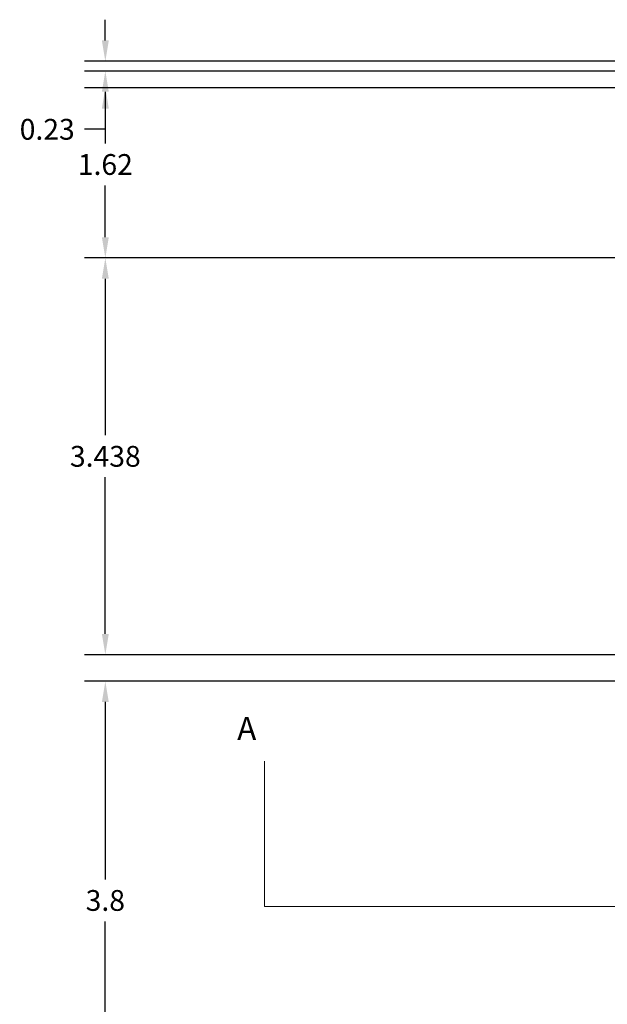
# Model space of a CAD drawing. Units: metres. Extents: x 2031 to 2061.8, y 1886.4 to 1909.8.
# Tile 4 of 10: x 2031 to 2036.1, y 1896.6 to 1905.1. Entities that reach past the tile are written whole.
import ezdxf

# ---------------------------------------------------------------- set-up
doc = ezdxf.new("R2010")
doc.units = ezdxf.units.M
doc.layers.add('A-ANNO-DIMS', color=2, linetype='Continuous', lineweight=18)
doc.layers.add('A-ANNO-SYMB', color=7, linetype='Continuous', lineweight=18)
doc.styles.get("Standard").update_dxf_attribs({"font": 'arial.ttf'})
doc.dimstyles.get("Standard").update_dxf_attribs({"dimtxt": 0.18, "dimasz": 0.18, "dimexe": 0.18, "dimexo": 0.0625, "dimgap": 0.09, "dimtad": 0, "dimtih": 1, "dimtoh": 1, "dimdec": 4, "dimzin": 0, "dimdsep": 46, "dimtxsty": 'Standard', "dimcen": 0.09, "dimadec": 0, "dimazin": 0, "dimtfac": 1, "dimtdec": 4, "dimtofl": 0, "dimtmove": 0, "dimatfit": 3, "dimfxl": 1, "dimtolj": 1, "dimtzin": 0, "dimarcsym": 0})

# ---------------------------------------------------------------- blocks, each defined once
blk = doc.blocks.new('*D51')
at = {"layer": 'A-ANNO-DIMS', "color": 0, "lineweight": -2, "transparency": 16777216}
for p, q in [((2036.9007, 1899.3712), (2031.5648, 1899.3712)), ((2031.7448, 1899.1912), (2031.7448, 1897.6532)), ((2031.7448, 1895.7512), (2031.7448, 1897.2892)), ((2036.9007, 1895.5712), (2031.5648, 1895.5712))]:
    blk.add_line(p, q, dxfattribs=at)
at = {"layer": 'A-ANNO-DIMS', "color": 0, "transparency": 16777216}
for points in [[(2031.7148, 1899.1912), (2031.7748, 1899.1912), (2031.7448, 1899.3712)], [(2031.7148, 1895.7512), (2031.7748, 1895.7512), (2031.7448, 1895.5712)]]:
    blk.add_solid(points, dxfattribs=at)
at = {"layer": 'Defpoints', "color": 0, "transparency": 16777216}
for p in [(2031.7448, 1899.3712), (2036.9632, 1899.3712), (2036.9632, 1895.5712)]:
    blk.add_point(p, dxfattribs=at)
at = {"layer": 'A-ANNO-DIMS', "color": 0, "transparency": 16777216, "insert": (2031.7448, 1897.4712), "char_height": 0.18, "attachment_point": 5}
blk.add_mtext('\\A1;3.8', dxfattribs=at)
blk = doc.blocks.new('*D52')
at = {"layer": 'A-ANNO-DIMS', "color": 0, "lineweight": -2, "transparency": 16777216}
for p, q in [((2036.1714, 1903.039), (2031.5648, 1903.039)), ((2031.7448, 1902.859), (2031.7448, 1901.5021)), ((2031.7448, 1899.7812), (2031.7448, 1901.1381)), ((2036.6707, 1899.6012), (2031.5648, 1899.6012))]:
    blk.add_line(p, q, dxfattribs=at)
at = {"layer": 'A-ANNO-DIMS', "color": 0, "transparency": 16777216}
for points in [[(2031.7148, 1902.859), (2031.7748, 1902.859), (2031.7448, 1903.039)], [(2031.7148, 1899.7812), (2031.7748, 1899.7812), (2031.7448, 1899.6012)]]:
    blk.add_solid(points, dxfattribs=at)
at = {"layer": 'Defpoints', "color": 0, "transparency": 16777216}
for p in [(2031.7448, 1903.039), (2036.2339, 1903.039), (2036.7332, 1899.6012)]:
    blk.add_point(p, dxfattribs=at)
at = {"layer": 'A-ANNO-DIMS', "color": 0, "transparency": 16777216, "insert": (2031.7448, 1901.3201), "char_height": 0.18, "attachment_point": 5}
blk.add_mtext('\\A1;3.438', dxfattribs=at)
blk = doc.blocks.new('*D53')
at = {"layer": 'A-ANNO-DIMS', "color": 0, "lineweight": -2, "transparency": 16777216}
for p, q in [((2036.1714, 1904.6594), (2031.5648, 1904.6594)), ((2031.7448, 1904.4794), (2031.7448, 1904.0311)), ((2031.7448, 1903.219), (2031.7448, 1903.6673)), ((2036.1714, 1903.039), (2031.5648, 1903.039))]:
    blk.add_line(p, q, dxfattribs=at)
at = {"layer": 'A-ANNO-DIMS', "color": 0, "transparency": 16777216}
for points in [[(2031.7148, 1904.4794), (2031.7748, 1904.4794), (2031.7448, 1904.6594)], [(2031.7148, 1903.219), (2031.7748, 1903.219), (2031.7448, 1903.039)]]:
    blk.add_solid(points, dxfattribs=at)
at = {"layer": 'Defpoints', "color": 0, "transparency": 16777216}
for p in [(2031.7448, 1904.6594), (2036.2339, 1904.6594), (2036.2339, 1903.039)]:
    blk.add_point(p, dxfattribs=at)
at = {"layer": 'A-ANNO-DIMS', "color": 0, "transparency": 16777216, "insert": (2031.7448, 1903.8492), "char_height": 0.18, "attachment_point": 5}
blk.add_mtext('\\A1;1.62', dxfattribs=at)
blk = doc.blocks.new('*D60')
at = {"layer": 'A-ANNO-DIMS', "color": 0, "lineweight": -2, "transparency": 16777216}
for p, q in [((2031.7448, 1904.9241), (2031.7448, 1905.1041)), ((2056.1614, 1904.7441), (2031.5648, 1904.7441)), ((2055.9314, 1904.5141), (2031.5648, 1904.5141)), ((2031.7448, 1904.3341), (2031.7448, 1904.1541)), ((2031.7448, 1904.1541), (2031.5648, 1904.1541))]:
    blk.add_line(p, q, dxfattribs=at)
at = {"layer": 'A-ANNO-DIMS', "color": 0, "transparency": 16777216}
for points in [[(2031.7148, 1904.9241), (2031.7748, 1904.9241), (2031.7448, 1904.7441)], [(2031.7148, 1904.3341), (2031.7748, 1904.3341), (2031.7448, 1904.5141)]]:
    blk.add_solid(points, dxfattribs=at)
at = {"layer": 'Defpoints', "color": 0, "transparency": 16777216}
for p in [(2056.2239, 1904.7441), (2031.7448, 1904.5141), (2055.9939, 1904.5141)]:
    blk.add_point(p, dxfattribs=at)
at = {"layer": 'A-ANNO-DIMS', "color": 0, "transparency": 16777216, "insert": (2031.241, 1904.1541), "char_height": 0.18, "attachment_point": 5}
blk.add_mtext('\\A1;0.23', dxfattribs=at)

msp = doc.modelspace()

# ---------------------------------------------------------------- linework, layer by layer
at = {"layer": 'A-ANNO-SYMB'}
for q in [(2033.1258, 1898.6774), (2060.0534, 1897.42)]:
    msp.add_line((2033.1258, 1897.42), q, dxfattribs=at)

# ---------------------------------------------------------------- texts
at = {"layer": 'A-ANNO-SYMB', "insert": (2032.8877, 1898.8613), "char_height": 0.2, "attachment_point": 7}
msp.add_mtext_dynamic_manual_height_columns('A', width=2.30233, gutter_width=12.5, heights=[0], dxfattribs=at)

# ---------------------------------------------------------------- dimensions: what is measured, and where the dimension line sits
at = {"layer": 'A-ANNO-DIMS'}
for base, p1, p2, override, picture, middle in [((2031.7448, 1904.5141), (2056.2239, 1904.7441), (2055.9939, 1904.5141), {"dimdec": 2, "dimlfac": 1, "dimrnd": 0, "dimzin": 0, "dimdsep": 46, "dimlunit": 2}, '*D60', (2031.241, 1904.1541)), ((2031.7448, 1904.6594), (2036.2339, 1903.039), (2036.2339, 1904.6594), {"dimdec": 2, "dimlfac": 1, "dimrnd": 0, "dimzin": 0, "dimdsep": 46, "dimlunit": 2}, '*D53', (2031.7448, 1903.8492)), ((2031.7448, 1903.039), (2036.7332, 1899.6012), (2036.2339, 1903.039), {"dimdec": 3, "dimlfac": 1, "dimrnd": 0, "dimzin": 0, "dimdsep": 46, "dimlunit": 2}, '*D52', (2031.7448, 1901.3201)), ((2031.7448, 1899.3712), (2036.9632, 1895.5712), (2036.9632, 1899.3712), {"dimdec": 1, "dimlfac": 1, "dimrnd": 0, "dimzin": 0, "dimdsep": 46, "dimlunit": 2}, '*D51', (2031.7448, 1897.4712))]:
    dim = msp.add_linear_dim(base=base, p1=p1, p2=p2, angle=90, dimstyle='Standard', override=override, dxfattribs=at)
    dim.commit()
    dim.dimension.update_dxf_attribs({"geometry": picture, "text_midpoint": middle})

doc.saveas('drawing.dxf')
